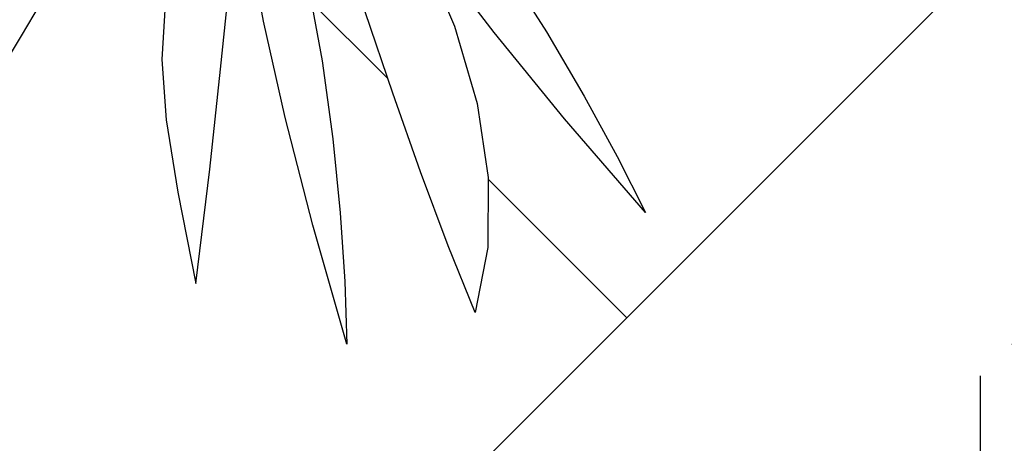
# Model space of a CAD drawing. Units: inches. Extents: x 3590 to 5167, y 65 to 1917.
# Tile 73 of 100: x 5046 to 5065, y 1765 to 1773. Entities that reach past the tile are written whole.
import ezdxf

# ---------------------------------------------------------------- set-up
doc = ezdxf.new("R2010")
doc.units = ezdxf.units.IN
for name, color, linetype, lineweight in [('A-ANNO-DIMS', 2, 'Continuous', 18), ('A-FLOR-PATT', 8, 'Continuous', 13), ('L-PLNT', 94, 'Continuous', 18)]:
    doc.layers.add(name, color=color, linetype=linetype, lineweight=lineweight)
doc.layers.add('DIENHOA', color=3, linetype='Continuous')
doc.styles.get("Standard").update_dxf_attribs({"font": 'arial.ttf'})
doc.dimstyles.new('ISO-25', dxfattribs={"dimtxt": 9, "dimasz": 2.5, "dimexe": 1.25, "dimexo": 0.625, "dimtad": 1, "dimdec": 1, "dimlunit": 3, "dimtxsty": 'Standard', "dimcen": 2.5, "dimadec": 0, "dimazin": 0, "dimtfac": 1, "dimtdec": 1, "dimtmove": 0, "dimatfit": 3, "dimfxl": 1, "dimarcsym": 0})

# ---------------------------------------------------------------- blocks, each defined once
blk = doc.blocks.new('Cay03_mb')
at = {"layer": 'DIENHOA'}
for p, q in [((135.85, -204.28), (162.8, -268.28)), ((113.06, -322.16), (90.79, -256.57)), ((162.8, -268.28), (180.96, -330.4)), ((135.38, -385.56), (113.06, -322.16)), ((180.96, -330.4), (190.01, -389.96)), ((157.6, -444.99), (135.38, -385.56)), ((190.01, -389.96), (189.65, -446.27)), ((179.55, -498.66), (157.6, -444.99)), ((189.65, -446.27), (179.55, -498.66))]:
    blk.add_line(p, q, dxfattribs=at)
for points in [[(23.69, -5.44), (-13.63, -87.94), (-41.14, -152.63), (-59.64, -205.04), (-69.94, -250.66), (-72.84, -295), (-69.17, -343.58), (-59.73, -401.89), (-45.32, -475.45)], [(-45.32, -475.45), (-34.09, -383.24), (-25.4, -302.82), (-18.34, -233.08), (-12.02, -172.9), (-5.55, -121.16), (1.96, -76.75), (11.41, -38.55), (23.69, -5.44)], [(316.49, -418.14), (251.44, -342.76), (194.84, -273.28), (146.52, -210.16), (106.33, -153.83), (74.11, -104.75), (49.71, -63.36), (32.95, -30.11), (23.69, -5.44)], [(23.69, -5.44), (74.94, -57.08), (121.78, -110.58), (164.32, -165.02), (202.67, -219.43), (236.95, -272.89), (267.27, -324.46), (293.75, -373.19), (316.49, -418.14)], [(-276.22, -424.43), (-227.35, -345.43), (-185.71, -276.08), (-150.05, -215.74), (-119.06, -163.76), (-91.49, -119.51), (-66.04, -82.35), (-41.43, -51.64), (-16.39, -26.73)], [(76.25, -524.2), (48.83, -428.48), (26.6, -341.67), (9.22, -264.1), (-3.63, -196.11), (-12.28, -138.04), (-17.07, -90.23), (-18.33, -53.01), (-16.39, -26.73)], [(-16.39, -26.73), (8.47, -95.11), (28.54, -163.33), (44.32, -230.59), (56.3, -296.08), (64.99, -358.99), (70.88, -418.52), (74.46, -473.86), (76.25, -524.2)]]:
    blk.add_lwpolyline(points, dxfattribs=at)
blk = doc.blocks.new('*D322')
at = {"layer": 'A-ANNO-DIMS', "color": 0, "lineweight": -2, "transparency": 16777216}
for p, q in [((5035.744, 1766.184), (5035.744, 1761.199)), ((5064.812, 1766.184), (5064.812, 1761.199)), ((5038.244, 1762.449), (5062.312, 1762.449)), ((5064.812, 1762.449), (5166.991, 1762.449))]:
    blk.add_line(p, q, dxfattribs=at)
at = {"layer": 'A-ANNO-DIMS', "color": 0, "transparency": 16777216}
for points in [[(5038.244, 1762.866), (5038.244, 1762.032), (5035.744, 1762.449)], [(5062.312, 1762.866), (5062.312, 1762.032), (5064.812, 1762.449)]]:
    blk.add_solid(points, dxfattribs=at)
at = {"layer": 'Defpoints', "color": 0, "transparency": 16777216}
for p in [(5035.744, 1766.809), (5064.812, 1766.809), (5064.812, 1762.449)]:
    blk.add_point(p, dxfattribs=at)
at = {"layer": 'A-ANNO-DIMS', "color": 0, "transparency": 16777216, "insert": (5117.152, 1767.669), "char_height": 9, "attachment_point": 5}
blk.add_mtext('PLANT 2\'-5" TYP.', dxfattribs=at)
blk = doc.blocks.new('*D323')
at = {"layer": 'A-ANNO-DIMS', "color": 0, "lineweight": -2, "transparency": 16777216}
for p, q in [((5069.172, 1795.216), (5069.172, 1874.95)), ((5065.437, 1795.216), (5070.422, 1795.216)), ((5069.172, 1769.309), (5069.172, 1792.716)), ((5065.437, 1766.809), (5070.422, 1766.809))]:
    blk.add_line(p, q, dxfattribs=at)
at = {"layer": 'A-ANNO-DIMS', "color": 0, "transparency": 16777216}
for points in [[(5068.756, 1792.716), (5069.589, 1792.716), (5069.172, 1795.216)], [(5068.756, 1769.309), (5069.589, 1769.309), (5069.172, 1766.809)]]:
    blk.add_solid(points, dxfattribs=at)
at = {"layer": 'Defpoints', "color": 0, "transparency": 16777216}
for p in [(5064.812, 1795.216), (5069.172, 1795.216), (5064.812, 1766.809)]:
    blk.add_point(p, dxfattribs=at)
at = {"layer": 'A-ANNO-DIMS', "color": 0, "transparency": 16777216, "insert": (5063.894, 1836.333), "char_height": 9, "attachment_point": 5, "rotation": 90}
blk.add_mtext('2\'-4 1/2" TYP.', dxfattribs=at)

msp = doc.modelspace()

# ---------------------------------------------------------------- hatches: boundary and pattern name
at = {"layer": 'A-FLOR-PATT', "transparency": 33554687}
h = msp.add_hatch(dxfattribs=at)
h.set_pattern_fill('AR-HBONE', color=256, scale=0.2)
h.set_pattern_definition([(45, (-588.972, 0), (0, 28.73682), [60.96, -20.32]), (135, (-574.604, 14.368), (3e-15, 28.73682), [60.96, -20.32])])
h.paths.add_polyline_path([(5071.274, 1796.999), (4933.274, 1796.999), (4933.274, 1753.999), (4962.774, 1753.999, -0.414214), (4928.774, 1719.999), (4933.274, 1718.999), (4933.274, 1334.999), (5071.274, 1334.999)])
h.paths.add_polyline_path([(4951.78, 1521.077), (4951.715, 1521.04), (4951.563, 1520.895)], flags=16)
h.paths.add_polyline_path([(4952.267, 1521.376), (4952.198, 1521.371), (4952.198, 1521.356)], flags=0)
h.paths.add_polyline_path([(4967.051, 1529.728), (4965.231, 1528.694), (4963.411, 1527.714), (4961.756, 1526.851), (4963.589, 1527.449), (4964.036, 1527.478), (4962.975, 1527.249), (4961.76, 1526.852), (4959.792, 1525.834), (4958.005, 1524.895), (4956.24, 1523.93), (4954.504, 1522.919), (4954.129, 1522.682), (4953.361, 1521.997), (4953.366, 1521.998), (4953.605, 1522.064), (4955.106, 1522.761), (4956.921, 1523.434), (4958.678, 1523.915), (4960.358, 1524.2), (4961.945, 1524.286), (4964.171, 1524.108), (4965.958, 1523.309), (4963.863, 1522.976), (4965.187, 1522.499), (4963.366, 1522.497), (4961.545, 1522.487), (4959.764, 1522.461), (4958.304, 1522.419), (4957.974, 1522.388), (4956.307, 1522.232), (4954.718, 1522.071), (4953.251, 1521.899), (4953.525, 1521.623), (4954.331, 1521.379), (4956.243, 1521.23), (4958.039, 1520.93), (4959.684, 1520.483), (4961.16, 1519.896), (4963.107, 1518.8), (4964.393, 1517.325), (4962.973, 1517.726), (4964.558, 1516.661), (4965.407, 1515.708), (4963.507, 1516.322), (4961.68, 1517.005), (4959.935, 1517.745), (4958.282, 1518.528), (4956.732, 1519.343), (4955.295, 1520.175), (4954.672, 1520.572), (4954.513, 1520.627), (4955.658, 1519.318), (4956.703, 1517.982), (4957.644, 1516.647), (4958.485, 1515.334), (4959.55, 1513.524), (4960.438, 1511.769), (4958.841, 1513.62), (4957.452, 1515.325), (4955.819, 1517.459), (4956.665, 1515.448), (4957.111, 1513.923), (4957.447, 1511.714), (4957.076, 1509.793), (4956.538, 1511.11), (4955.992, 1512.569), (4955.444, 1514.125), (4954.898, 1515.735), (4954.357, 1517.356), (4953.824, 1518.943), (4953.305, 1520.452), (4953.065, 1521.116), (4952.971, 1521.146), (4952.949, 1521.086), (4952.73, 1520.199), (4953.37, 1518.024), (4953.757, 1516.373), (4954.051, 1514.765), (4954.264, 1513.221), (4954.471, 1511.131), (4954.497, 1510.402), (4954.409, 1511.76), (4954.264, 1513.221), (4954.051, 1514.765), (4953.757, 1516.373), (4953.37, 1518.024), (4952.877, 1519.698), (4952.716, 1520.141), (4952.533, 1519.059), (4952.374, 1517.789), (4952.219, 1516.312), (4952.046, 1514.6), (4951.833, 1512.626), (4951.557, 1510.363), (4951.203, 1512.168), (4950.852, 1514.339), (4950.985, 1516.376), (4951.66, 1518.286), (4952.593, 1520.481), (4952.357, 1521.13), (4951.855, 1520.328), (4950.839, 1518.908), (4949.777, 1517.587), (4948.916, 1516.617), (4948.111, 1515.256), (4947.089, 1513.554), (4945.889, 1511.615), (4946.326, 1513.402), (4946.562, 1514.249), (4945.528, 1513.327), (4944.581, 1512.531), (4946.018, 1514.508), (4947.204, 1516.048), (4947.893, 1517.313), (4949.307, 1518.764), (4950.414, 1519.767), (4950.451, 1519.806), (4952.267, 1521.376), (4951.645, 1521.493), (4950.404, 1521.18), (4948.044, 1520.359), (4946.119, 1519.452), (4944.572, 1518.475), (4943.35, 1517.443), (4941.997, 1515.92), (4941.661, 1515.275), (4942.813, 1516.99), (4944.572, 1518.475), (4946.119, 1519.452), (4948.044, 1520.359), (4950.404, 1521.18), (4951.645, 1521.493), (4949.647, 1521.868), (4948.6, 1521.756), (4947.126, 1521.57), (4945.42, 1521.348), (4943.45, 1521.105), (4941.183, 1520.856), (4942.86, 1521.613), (4943.873, 1522.03), (4942.952, 1521.909), (4941.41, 1521.485), (4939.543, 1520.67), (4938.968, 1520.226), (4940.733, 1521.299), (4942.952, 1521.909), (4943.702, 1522.008), (4945.894, 1522.7), (4947.565, 1522.714), (4948.921, 1522.566), (4951.131, 1522.183), (4950.971, 1522.297), (4948.129, 1523.006), (4946.035, 1523.707), (4944.232, 1524.521), (4942.707, 1525.461), (4941.444, 1526.537), (4940.43, 1527.761), (4939.649, 1529.143), (4941.421, 1528.122), (4943.147, 1527.132), (4944.841, 1526.175), (4946.514, 1525.25), (4948.179, 1524.359), (4948.365, 1524.263), (4946.475, 1526.045), (4945.181, 1527.54), (4944.19, 1529.033), (4943.496, 1530.54), (4943.278, 1531.36), (4942.498, 1531.919), (4943.114, 1531.762), (4942.959, 1533.659), (4944.14, 1531.989), (4944.612, 1531.323), (4946.202, 1530.463), (4947.486, 1529.509), (4948.79, 1528.226), (4950.368, 1526.237), (4949.485, 1528.155), (4948.851, 1530.123), (4948.491, 1532.041), (4948.381, 1533.918), (4948.501, 1535.76), (4948.827, 1537.573), (4949.418, 1535.565), (4949.957, 1533.569), (4950.464, 1531.586), (4950.961, 1529.617), (4951.391, 1527.954), (4951.724, 1530.687), (4952.201, 1532.58), (4952.889, 1534.33), (4953.77, 1535.951), (4954.827, 1537.46), (4954.521, 1535.39), (4954.273, 1533.937), (4955.58, 1535.663), (4956.748, 1536.739), (4956.159, 1534.78), (4955.589, 1532.873), (4955.043, 1531.006), (4954.525, 1529.166), (4954.038, 1527.341), (4953.638, 1525.733), (4953.611, 1525.586), (4953.398, 1524.166), (4953.382, 1524.009), (4954.07, 1525.476), (4954.912, 1527.022), (4956.136, 1528.894), (4957.847, 1530.577), (4959.376, 1531.54), (4958.256, 1530.104), (4957.143, 1528.663), (4956.066, 1527.243), (4955.056, 1525.871), (4954.141, 1524.571), (4953.352, 1523.372), (4953.311, 1523.303), (4953.273, 1522.925), (4953.261, 1522.382), (4954.103, 1523.373), (4954.63, 1524.284), (4955.961, 1526.358), (4957.23, 1528.13), (4958.421, 1529.609), (4960.037, 1531.368), (4961.374, 1532.375), (4962.101, 1532.77), (4961.07, 1531.061), (4959.987, 1529.438), (4958.869, 1527.908), (4958.15, 1527.007), (4959.803, 1528.003), (4961.589, 1528.793), (4963.391, 1529.328), (4965.211, 1529.632)], flags=16)
h.paths.add_polyline_path([(4962.944, 1523.182), (4961.107, 1523.422), (4960.392, 1523.362), (4962.35, 1523.331)], flags=0)
h.paths.add_polyline_path([(5049.541, 1584.551), (5049.476, 1584.515), (5049.325, 1584.37)], flags=16)
h.paths.add_polyline_path([(5050.028, 1584.851), (5049.959, 1584.845), (5049.959, 1584.83)], flags=0)
h.paths.add_polyline_path([(5042.333, 1581.949), (5043.88, 1582.926), (5045.806, 1583.833), (5048.165, 1584.654), (5049.406, 1584.967), (5047.408, 1585.342), (5046.361, 1585.231), (5044.888, 1585.044), (5043.181, 1584.822), (5041.211, 1584.579), (5038.944, 1584.33), (5040.622, 1585.087), (5041.634, 1585.504), (5040.713, 1585.383), (5039.171, 1584.959), (5037.304, 1584.144), (5036.729, 1583.7), (5038.494, 1584.773), (5040.713, 1585.383), (5041.463, 1585.482), (5043.655, 1586.174), (5045.326, 1586.188), (5046.682, 1586.04), (5048.893, 1585.657), (5048.732, 1585.771), (5045.891, 1586.48), (5043.796, 1587.181), (5041.994, 1587.996), (5040.468, 1588.935), (5039.205, 1590.011), (5038.191, 1591.235), (5037.41, 1592.617), (5039.182, 1591.596), (5040.909, 1590.607), (5042.602, 1589.649), (5044.275, 1588.724), (5045.94, 1587.833), (5046.126, 1587.738), (5044.237, 1589.519), (5042.942, 1591.015), (5041.952, 1592.508), (5041.257, 1594.014), (5041.039, 1594.834), (5040.26, 1595.393), (5040.875, 1595.237), (5040.721, 1597.133), (5041.901, 1595.463), (5042.373, 1594.798), (5043.963, 1593.938), (5045.247, 1592.983), (5046.552, 1591.701), (5048.129, 1589.712), (5047.247, 1591.63), (5046.613, 1593.597), (5046.252, 1595.515), (5046.142, 1597.392), (5046.262, 1599.234), (5046.588, 1601.047), (5047.179, 1599.039), (5047.718, 1597.043), (5048.225, 1595.06), (5048.722, 1593.091), (5049.152, 1591.429), (5049.485, 1594.161), (5049.962, 1596.054), (5050.65, 1597.804), (5051.532, 1599.425), (5052.589, 1600.934), (5052.283, 1598.864), (5052.034, 1597.411), (5053.341, 1599.137), (5054.509, 1600.213), (5053.92, 1598.254), (5053.35, 1596.348), (5052.805, 1594.48), (5052.286, 1592.64), (5051.799, 1590.815), (5051.4, 1589.207), (5051.373, 1589.06), (5051.159, 1587.64), (5051.143, 1587.483), (5051.831, 1588.95), (5052.673, 1590.496), (5053.898, 1592.368), (5055.608, 1594.051), (5057.137, 1595.014), (5056.017, 1593.578), (5054.904, 1592.137), (5053.828, 1590.717), (5052.817, 1589.345), (5051.902, 1588.046), (5051.113, 1586.846), (5051.072, 1586.777), (5051.034, 1586.399), (5051.022, 1585.856), (5051.864, 1586.847), (5052.391, 1587.758), (5053.723, 1589.832), (5054.991, 1591.604), (5056.182, 1593.083), (5057.798, 1594.842), (5059.135, 1595.849), (5059.863, 1596.244), (5058.831, 1594.535), (5057.749, 1592.912), (5056.63, 1591.382), (5055.912, 1590.482), (5057.564, 1591.477), (5059.35, 1592.267), (5061.152, 1592.802), (5062.972, 1593.106), (5064.812, 1593.203), (5062.992, 1592.169), (5061.172, 1591.188), (5059.518, 1590.325), (5061.35, 1590.924), (5061.797, 1590.952), (5060.737, 1590.723), (5059.521, 1590.326), (5057.553, 1589.308), (5055.766, 1588.369), (5054.002, 1587.404), (5052.265, 1586.393), (5051.891, 1586.156), (5051.122, 1585.471), (5051.127, 1585.472), (5051.366, 1585.538), (5052.867, 1586.235), (5054.682, 1586.908), (5056.439, 1587.389), (5058.12, 1587.675), (5059.706, 1587.76), (5061.933, 1587.583), (5063.719, 1586.783), (5061.624, 1586.45), (5062.949, 1585.973), (5061.127, 1585.971), (5059.307, 1585.961), (5057.525, 1585.935), (5056.065, 1585.893), (5055.735, 1585.862), (5054.068, 1585.707), (5052.479, 1585.546), (5051.012, 1585.373), (5051.286, 1585.097), (5052.092, 1584.853), (5054.004, 1584.704), (5055.8, 1584.404), (5057.446, 1583.958), (5058.921, 1583.37), (5060.868, 1582.274), (5062.154, 1580.799), (5060.734, 1581.2), (5062.32, 1580.135), (5063.168, 1579.182), (5061.269, 1579.796), (5059.441, 1580.479), (5057.696, 1581.219), (5056.043, 1582.003), (5054.493, 1582.817), (5053.057, 1583.649), (5052.433, 1584.047), (5052.274, 1584.101), (5053.42, 1582.793), (5054.464, 1581.457), (5055.405, 1580.121), (5056.247, 1578.809), (5057.311, 1576.998), (5058.199, 1575.244), (5056.602, 1577.094), (5055.213, 1578.799), (5053.58, 1580.933), (5054.427, 1578.922), (5054.872, 1577.397), (5055.208, 1575.189), (5054.838, 1573.267), (5054.299, 1574.584), (5053.754, 1576.043), (5053.206, 1577.599), (5052.659, 1579.209), (5052.118, 1580.83), (5051.585, 1582.417), (5051.066, 1583.927), (5050.826, 1584.59), (5050.733, 1584.62), (5050.711, 1584.561), (5050.491, 1583.673), (5051.131, 1581.498), (5051.518, 1579.847), (5051.813, 1578.24), (5052.026, 1576.695), (5052.233, 1574.605), (5052.258, 1573.876), (5052.17, 1575.234), (5052.026, 1576.695), (5051.813, 1578.24), (5051.518, 1579.847), (5051.131, 1581.498), (5050.638, 1583.172), (5050.477, 1583.615), (5050.294, 1582.533), (5050.136, 1581.263), (5049.981, 1579.786), (5049.807, 1578.074), (5049.594, 1576.1), (5049.318, 1573.837), (5048.965, 1575.642), (5048.613, 1577.813), (5048.747, 1579.85), (5049.421, 1581.76), (5050.354, 1583.955), (5050.118, 1584.604), (5049.616, 1583.802), (5048.6, 1582.382), (5047.538, 1581.061), (5046.677, 1580.091), (5045.872, 1578.73), (5044.85, 1577.028), (5043.651, 1575.089), (5044.087, 1576.877), (5044.324, 1577.723), (5043.289, 1576.801), (5042.342, 1576.005), (5043.779, 1577.982), (5044.966, 1579.522), (5045.655, 1580.787), (5047.068, 1582.239), (5048.175, 1583.241), (5048.213, 1583.28), (5050.028, 1584.851), (5049.406, 1584.967), (5048.165, 1584.654), (5045.806, 1583.833), (5043.88, 1582.926), (5042.333, 1581.949), (5041.111, 1580.917), (5039.758, 1579.394), (5039.423, 1578.749), (5040.575, 1580.464)], flags=16)
h.paths.add_polyline_path([(4954.799, 1533.12), (4954.262, 1532.079), (4953.831, 1530.935), (4953.505, 1529.636), (4953.283, 1528.133), (4953.167, 1526.376), (4953.156, 1524.315), (4953.277, 1521.236), (4952.802, 1521.842), (4951.557, 1521.998), (4950.976, 1521.961), (4952.661, 1521.941), (4952.802, 1521.842), (4953.152, 1523.593), (4953.167, 1526.376), (4953.283, 1528.133), (4953.609, 1530.346), (4954.456, 1532.592)], flags=0)
h.paths.add_polyline_path([(5050.563, 1585.316), (5049.318, 1585.472), (5048.737, 1585.435), (5050.422, 1585.415), (5050.563, 1585.316), (5050.914, 1587.067), (5050.928, 1589.851), (5051.045, 1591.607), (5051.371, 1593.82), (5052.217, 1596.066), (5052.56, 1596.594), (5052.024, 1595.554), (5051.592, 1594.409), (5051.266, 1593.11), (5051.045, 1591.607), (5050.928, 1589.851), (5050.918, 1587.789), (5051.038, 1584.71)], flags=0)
h.paths.add_polyline_path([(5058.153, 1586.836), (5060.111, 1586.805), (5060.705, 1586.656), (5058.868, 1586.896)], flags=0)
h.paths.add_polyline_path([(5049.541, 1430.936), (5049.476, 1430.9), (5049.325, 1430.755)], flags=16)
h.paths.add_polyline_path([(5050.028, 1431.236), (5049.959, 1431.231), (5049.959, 1431.215)], flags=0)
h.paths.add_polyline_path([(5046.588, 1447.432), (5047.179, 1445.425), (5047.718, 1443.429), (5048.225, 1441.446), (5048.722, 1439.476), (5049.152, 1437.814), (5049.485, 1440.546), (5049.962, 1442.439), (5050.65, 1444.189), (5051.532, 1445.811), (5052.589, 1447.319), (5052.283, 1445.249), (5052.034, 1443.796), (5053.341, 1445.522), (5054.509, 1446.598), (5053.92, 1444.64), (5053.35, 1442.733), (5052.805, 1440.865), (5052.286, 1439.025), (5051.799, 1437.201), (5051.4, 1435.592), (5051.373, 1435.445), (5051.159, 1434.025), (5051.143, 1433.868), (5051.831, 1435.335), (5052.673, 1436.881), (5053.898, 1438.753), (5055.608, 1440.436), (5057.137, 1441.4), (5056.017, 1439.963), (5054.904, 1438.522), (5053.828, 1437.102), (5052.817, 1435.73), (5051.902, 1434.431), (5051.113, 1433.231), (5051.072, 1433.162), (5051.034, 1432.784), (5051.022, 1432.242), (5051.864, 1433.232), (5052.391, 1434.143), (5053.723, 1436.217), (5054.991, 1437.989), (5056.182, 1439.468), (5057.798, 1441.227), (5059.135, 1442.235), (5059.863, 1442.629), (5058.831, 1440.921), (5057.749, 1439.298), (5056.63, 1437.767), (5055.912, 1436.867), (5057.564, 1437.863), (5059.35, 1438.652), (5061.152, 1439.187), (5062.972, 1439.491), (5064.812, 1439.588), (5062.992, 1438.554), (5061.172, 1437.573), (5059.518, 1436.71), (5061.35, 1437.309), (5061.797, 1437.337), (5060.737, 1437.108), (5059.521, 1436.711), (5057.553, 1435.693), (5055.766, 1434.754), (5054.002, 1433.789), (5052.265, 1432.778), (5051.891, 1432.541), (5051.122, 1431.856), (5051.127, 1431.857), (5051.366, 1431.923), (5052.867, 1432.62), (5054.682, 1433.293), (5056.439, 1433.775), (5058.12, 1434.06), (5059.706, 1434.145), (5061.933, 1433.968), (5063.719, 1433.168), (5061.624, 1432.835), (5062.949, 1432.358), (5061.127, 1432.357), (5059.307, 1432.346), (5057.525, 1432.32), (5056.065, 1432.278), (5055.735, 1432.248), (5054.068, 1432.092), (5052.479, 1431.931), (5051.012, 1431.759), (5051.286, 1431.482), (5052.092, 1431.238), (5054.004, 1431.089), (5055.8, 1430.789), (5057.446, 1430.343), (5058.921, 1429.755), (5060.868, 1428.66), (5062.154, 1427.185), (5060.734, 1427.585), (5062.32, 1426.52), (5063.168, 1425.567), (5061.269, 1426.181), (5059.441, 1426.865), (5057.696, 1427.604), (5056.043, 1428.388), (5054.493, 1429.202), (5053.057, 1430.034), (5052.433, 1430.432), (5052.274, 1430.487), (5053.42, 1429.178), (5054.464, 1427.842), (5055.405, 1426.506), (5056.247, 1425.194), (5057.311, 1423.383), (5058.199, 1421.629), (5056.602, 1423.479), (5055.213, 1425.184), (5053.58, 1427.318), (5054.427, 1425.307), (5054.872, 1423.782), (5055.208, 1421.574), (5054.838, 1419.652), (5054.299, 1420.97), (5053.754, 1422.428), (5053.206, 1423.984), (5052.659, 1425.595), (5052.118, 1427.215), (5051.585, 1428.802), (5051.066, 1430.312), (5050.826, 1430.975), (5050.733, 1431.005), (5050.711, 1430.946), (5050.491, 1430.058), (5051.131, 1427.883), (5051.518, 1426.232), (5051.813, 1424.625), (5052.026, 1423.081), (5052.233, 1420.991), (5052.258, 1420.261), (5052.17, 1421.619), (5052.026, 1423.081), (5051.813, 1424.625), (5051.518, 1426.232), (5051.131, 1427.883), (5050.638, 1429.558), (5050.477, 1430.001), (5050.294, 1428.918), (5050.136, 1427.648), (5049.981, 1426.171), (5049.807, 1424.459), (5049.594, 1422.485), (5049.318, 1420.222), (5048.965, 1422.028), (5048.613, 1424.199), (5048.747, 1426.235), (5049.421, 1428.146), (5050.354, 1430.34), (5050.118, 1430.989), (5049.616, 1430.187), (5048.6, 1428.768), (5047.538, 1427.446), (5046.677, 1426.477), (5045.872, 1425.116), (5044.85, 1423.413), (5043.651, 1421.474), (5044.087, 1423.262), (5044.324, 1424.109), (5043.289, 1423.186), (5042.342, 1422.391), (5043.779, 1424.368), (5044.966, 1425.907), (5045.655, 1427.173), (5047.068, 1428.624), (5048.175, 1429.627), (5048.213, 1429.666), (5050.028, 1431.236), (5049.406, 1431.353), (5048.165, 1431.039), (5045.806, 1430.218), (5043.88, 1429.311), (5042.333, 1428.334), (5041.111, 1427.302), (5039.758, 1425.779), (5039.423, 1425.134), (5040.575, 1426.849), (5042.333, 1428.334), (5043.88, 1429.311), (5045.806, 1430.218), (5048.165, 1431.039), (5049.406, 1431.353), (5047.408, 1431.727), (5046.361, 1431.616), (5044.888, 1431.429), (5043.181, 1431.207), (5041.211, 1430.964), (5038.944, 1430.715), (5040.622, 1431.472), (5041.634, 1431.89), (5040.713, 1431.769), (5039.171, 1431.345), (5037.304, 1430.53), (5036.729, 1430.085), (5038.494, 1431.158), (5040.713, 1431.769), (5041.463, 1431.867), (5043.655, 1432.559), (5045.326, 1432.573), (5046.682, 1432.425), (5048.893, 1432.042), (5048.732, 1432.156), (5045.891, 1432.865), (5043.796, 1433.566), (5041.994, 1434.381), (5040.468, 1435.321), (5039.205, 1436.396), (5038.191, 1437.62), (5037.41, 1439.002), (5039.182, 1437.982), (5040.909, 1436.992), (5042.602, 1436.034), (5044.275, 1435.109), (5045.94, 1434.218), (5046.126, 1434.123), (5044.237, 1435.904), (5042.942, 1437.4), (5041.952, 1438.893), (5041.257, 1440.399), (5041.039, 1441.219), (5040.26, 1441.778), (5040.875, 1441.622), (5040.721, 1443.518), (5041.901, 1441.848), (5042.373, 1441.183), (5043.963, 1440.323), (5045.247, 1439.369), (5046.552, 1438.086), (5048.129, 1436.097), (5047.247, 1438.015), (5046.613, 1439.982), (5046.252, 1441.901), (5046.142, 1443.778), (5046.262, 1445.619)], flags=16)
h.paths.add_polyline_path([(5052.382, 1444.255), (5051.623, 1442.78), (5052.024, 1441.939), (5052.56, 1442.98)], flags=0)
h.paths.add_polyline_path([(5050.563, 1431.701), (5049.318, 1431.857), (5048.737, 1431.821), (5050.422, 1431.8)], flags=0)
h.paths.add_polyline_path([(5058.153, 1433.221), (5060.111, 1433.19), (5060.705, 1433.041), (5058.868, 1433.281)], flags=0)
h.paths.add_polyline_path([(5049.541, 1352.285), (5049.476, 1352.249), (5049.325, 1352.104)], flags=16)
h.paths.add_polyline_path([(5050.028, 1352.585), (5049.959, 1352.58), (5049.959, 1352.564)], flags=0)
h.paths.add_polyline_path([(5046.588, 1368.781), (5047.179, 1366.774), (5047.718, 1364.778), (5048.225, 1362.795), (5048.722, 1360.825), (5049.152, 1359.163), (5049.485, 1361.896), (5049.962, 1363.789), (5050.65, 1365.538), (5051.532, 1367.16), (5052.589, 1368.669), (5052.283, 1366.598), (5052.034, 1365.145), (5053.341, 1366.871), (5054.509, 1367.947), (5053.92, 1365.989), (5053.35, 1364.082), (5052.805, 1362.214), (5052.286, 1360.374), (5051.799, 1358.55), (5051.4, 1356.942), (5051.373, 1356.794), (5051.159, 1355.374), (5051.143, 1355.218), (5051.831, 1356.684), (5052.673, 1358.23), (5053.898, 1360.102), (5055.608, 1361.786), (5057.137, 1362.749), (5056.017, 1361.313), (5054.904, 1359.872), (5053.828, 1358.452), (5052.817, 1357.079), (5051.902, 1355.78), (5051.113, 1354.581), (5051.072, 1354.512), (5051.034, 1354.133), (5051.022, 1353.591), (5051.864, 1354.581), (5052.391, 1355.492), (5053.723, 1357.566), (5054.991, 1359.338), (5056.182, 1360.817), (5057.798, 1362.577), (5059.135, 1363.584), (5059.863, 1363.979), (5058.831, 1362.27), (5057.749, 1360.647), (5056.63, 1359.117), (5055.912, 1358.216), (5057.564, 1359.212), (5059.35, 1360.001), (5061.152, 1360.536), (5062.972, 1360.841), (5064.812, 1360.937), (5062.992, 1359.903), (5061.172, 1358.923), (5059.518, 1358.059), (5061.35, 1358.658), (5061.797, 1358.687), (5060.737, 1358.458), (5059.521, 1358.061), (5057.553, 1357.043), (5055.766, 1356.103), (5054.002, 1355.138), (5052.265, 1354.127), (5051.891, 1353.89), (5051.122, 1353.206), (5051.127, 1353.206), (5051.366, 1353.272), (5052.867, 1353.969), (5054.682, 1354.643), (5056.439, 1355.124), (5058.12, 1355.409), (5059.706, 1355.495), (5061.933, 1355.317), (5063.719, 1354.518), (5061.624, 1354.184), (5062.949, 1353.708), (5061.127, 1353.706), (5059.307, 1353.695), (5057.525, 1353.669), (5056.065, 1353.627), (5055.735, 1353.597), (5054.068, 1353.441), (5052.479, 1353.28), (5051.012, 1353.108), (5051.286, 1352.831), (5052.092, 1352.587), (5054.004, 1352.439), (5055.8, 1352.138), (5057.446, 1351.692), (5058.921, 1351.104), (5060.868, 1350.009), (5062.154, 1348.534), (5060.734, 1348.935), (5062.32, 1347.869), (5063.168, 1346.916), (5061.269, 1347.53), (5059.441, 1348.214), (5057.696, 1348.954), (5056.043, 1349.737), (5054.493, 1350.551), (5053.057, 1351.383), (5052.433, 1351.781), (5052.274, 1351.836), (5053.42, 1350.527), (5054.464, 1349.191), (5055.405, 1347.855), (5056.247, 1346.543), (5057.311, 1344.733), (5058.199, 1342.978), (5056.602, 1344.828), (5055.213, 1346.534), (5053.58, 1348.667), (5054.427, 1346.656), (5054.872, 1345.132), (5055.208, 1342.923), (5054.838, 1341.002), (5054.299, 1342.319), (5053.754, 1343.778), (5053.206, 1345.334), (5052.659, 1346.944), (5052.118, 1348.564), (5051.585, 1350.151), (5051.066, 1351.661), (5050.826, 1352.324), (5050.733, 1352.355), (5050.711, 1352.295), (5050.491, 1351.408), (5051.131, 1349.232), (5051.518, 1347.581), (5051.813, 1345.974), (5052.026, 1344.43), (5052.233, 1342.34), (5052.258, 1341.61), (5052.17, 1342.969), (5052.026, 1344.43), (5051.813, 1345.974), (5051.518, 1347.581), (5051.131, 1349.232), (5050.638, 1350.907), (5050.477, 1351.35), (5050.294, 1350.267), (5050.136, 1348.997), (5049.981, 1347.52), (5049.807, 1345.809), (5049.594, 1343.835), (5049.318, 1341.571), (5048.965, 1343.377), (5048.613, 1345.548), (5048.747, 1347.585), (5049.421, 1349.495), (5050.354, 1351.689), (5050.118, 1352.339), (5049.616, 1351.536), (5048.6, 1350.117), (5047.538, 1348.795), (5046.677, 1347.826), (5045.872, 1346.465), (5044.85, 1344.763), (5043.651, 1342.824), (5044.087, 1344.611), (5044.324, 1345.458), (5043.289, 1344.535), (5042.342, 1343.74), (5043.779, 1345.717), (5044.966, 1347.256), (5045.655, 1348.522), (5047.068, 1349.973), (5048.175, 1350.976), (5048.213, 1351.015), (5050.028, 1352.585), (5049.406, 1352.702), (5048.165, 1352.388), (5045.806, 1351.567), (5043.88, 1350.661), (5042.333, 1349.683), (5041.111, 1348.651), (5039.758, 1347.128), (5039.423, 1346.483), (5040.575, 1348.198), (5042.333, 1349.683), (5043.88, 1350.661), (5045.806, 1351.567), (5048.165, 1352.388), (5049.406, 1352.702), (5047.408, 1353.076), (5046.361, 1352.965), (5044.888, 1352.779), (5043.181, 1352.556), (5041.211, 1352.313), (5038.944, 1352.065), (5040.622, 1352.821), (5041.634, 1353.239), (5040.713, 1353.118), (5039.171, 1352.694), (5037.304, 1351.879), (5036.729, 1351.434), (5038.494, 1352.508), (5040.713, 1353.118), (5041.463, 1353.216), (5043.655, 1353.909), (5045.326, 1353.923), (5046.682, 1353.774), (5048.893, 1353.391), (5048.732, 1353.506), (5045.891, 1354.214), (5043.796, 1354.915), (5041.994, 1355.73), (5040.468, 1356.67), (5039.205, 1357.746), (5038.191, 1358.969), (5037.41, 1360.352), (5039.182, 1359.331), (5040.909, 1358.341), (5042.602, 1357.383), (5044.275, 1356.458), (5045.94, 1355.567), (5046.126, 1355.472), (5044.237, 1357.253), (5042.942, 1358.749), (5041.952, 1360.242), (5041.257, 1361.748), (5041.039, 1362.568), (5040.26, 1363.128), (5040.875, 1362.971), (5040.721, 1364.867), (5041.901, 1363.197), (5042.373, 1362.532), (5043.963, 1361.672), (5045.247, 1360.718), (5046.552, 1359.435), (5048.129, 1357.446), (5047.247, 1359.364), (5046.613, 1361.331), (5046.252, 1363.25), (5046.142, 1365.127), (5046.262, 1366.969)], flags=16)
h.paths.add_polyline_path([(5052.382, 1365.604), (5051.623, 1364.129), (5052.024, 1363.288), (5052.56, 1364.329)], flags=0)
h.paths.add_polyline_path([(4951.78, 1698.041), (4951.715, 1698.005), (4951.563, 1697.859)], flags=16)
h.paths.add_polyline_path([(4952.267, 1698.341), (4952.198, 1698.335), (4952.198, 1698.32)], flags=0)
h.paths.add_polyline_path([(4957.076, 1686.757), (4956.538, 1688.074), (4955.992, 1689.533), (4955.444, 1691.089), (4954.898, 1692.699), (4954.357, 1694.32), (4953.824, 1695.907), (4953.305, 1697.417), (4953.065, 1698.08), (4952.971, 1698.11), (4952.949, 1698.051), (4952.73, 1697.163), (4953.37, 1694.988), (4953.757, 1693.337), (4954.051, 1691.729), (4954.264, 1690.185), (4954.471, 1688.095), (4954.497, 1687.366), (4954.409, 1688.724), (4954.264, 1690.185), (4954.051, 1691.729), (4953.757, 1693.337), (4953.37, 1694.988), (4952.877, 1696.662), (4952.716, 1697.105), (4952.533, 1696.023), (4952.374, 1694.753), (4952.219, 1693.276), (4952.046, 1691.564), (4951.833, 1689.59), (4951.557, 1687.327), (4951.203, 1689.132), (4950.852, 1691.303), (4950.985, 1693.34), (4951.66, 1695.25), (4952.593, 1697.445), (4952.357, 1698.094), (4951.855, 1697.292), (4950.839, 1695.872), (4949.777, 1694.551), (4948.916, 1693.581), (4948.111, 1692.22), (4947.089, 1690.518), (4945.889, 1688.579), (4946.326, 1690.366), (4946.562, 1691.213), (4945.528, 1690.291), (4944.581, 1689.495), (4946.018, 1691.472), (4947.204, 1693.012), (4947.893, 1694.277), (4949.307, 1695.729), (4950.414, 1696.731), (4950.451, 1696.77), (4952.267, 1698.341), (4951.645, 1698.457), (4950.404, 1698.144), (4948.044, 1697.323), (4946.119, 1696.416), (4944.572, 1695.439), (4943.35, 1694.407), (4941.997, 1692.884), (4941.661, 1692.239), (4942.813, 1693.954), (4944.572, 1695.439), (4946.119, 1696.416), (4948.044, 1697.323), (4950.404, 1698.144), (4951.645, 1698.457), (4949.647, 1698.832), (4948.6, 1698.72), (4947.126, 1698.534), (4945.42, 1698.312), (4943.45, 1698.069), (4941.183, 1697.82), (4942.86, 1698.577), (4943.873, 1698.994), (4942.952, 1698.873), (4941.41, 1698.449), (4939.543, 1697.634), (4938.968, 1697.19), (4940.733, 1698.263), (4942.952, 1698.873), (4943.702, 1698.972), (4945.894, 1699.664), (4947.565, 1699.678), (4948.921, 1699.53), (4951.131, 1699.147), (4950.971, 1699.261), (4948.129, 1699.97), (4946.035, 1700.671), (4944.232, 1701.486), (4942.707, 1702.425), (4941.444, 1703.501), (4940.43, 1704.725), (4939.649, 1706.107), (4941.421, 1705.086), (4943.147, 1704.097), (4944.841, 1703.139), (4946.514, 1702.214), (4948.179, 1701.323), (4948.365, 1701.227), (4946.475, 1703.009), (4945.181, 1704.505), (4944.19, 1705.997), (4943.496, 1707.504), (4943.278, 1708.324), (4942.498, 1708.883), (4943.114, 1708.727), (4942.959, 1710.623), (4944.14, 1708.953), (4944.612, 1708.287), (4946.202, 1707.428), (4947.486, 1706.473), (4948.79, 1705.191), (4950.368, 1703.202), (4949.485, 1705.12), (4948.851, 1707.087), (4948.491, 1709.005), (4948.381, 1710.882), (4948.501, 1712.724), (4948.827, 1714.537), (4949.418, 1712.529), (4949.957, 1710.533), (4950.464, 1708.55), (4950.961, 1706.581), (4951.391, 1704.919), (4951.724, 1707.651), (4952.201, 1709.544), (4952.889, 1711.294), (4953.77, 1712.915), (4954.827, 1714.424), (4954.521, 1712.354), (4954.273, 1710.901), (4955.58, 1712.627), (4956.748, 1713.703), (4956.159, 1711.744), (4955.589, 1709.837), (4955.043, 1707.97), (4954.525, 1706.13), (4954.038, 1704.305), (4953.638, 1702.697), (4953.611, 1702.55), (4953.398, 1701.13), (4953.382, 1700.973), (4954.07, 1702.44), (4954.912, 1703.986), (4956.136, 1705.858), (4957.847, 1707.541), (4959.376, 1708.504), (4958.256, 1707.068), (4957.143, 1705.627), (4956.066, 1704.207), (4955.056, 1702.835), (4954.141, 1701.536), (4953.352, 1700.336), (4953.311, 1700.267), (4953.273, 1699.889), (4953.261, 1699.346), (4954.103, 1700.337), (4954.63, 1701.248), (4955.961, 1703.322), (4957.23, 1705.094), (4958.421, 1706.573), (4960.037, 1708.332), (4961.374, 1709.339), (4962.101, 1709.734), (4961.07, 1708.025), (4959.987, 1706.402), (4958.869, 1704.872), (4958.15, 1703.972), (4959.803, 1704.967), (4961.589, 1705.757), (4963.391, 1706.292), (4965.211, 1706.596), (4967.051, 1706.692), (4965.231, 1705.659), (4963.411, 1704.678), (4961.756, 1703.815), (4963.589, 1704.413), (4964.036, 1704.442), (4962.975, 1704.213), (4961.76, 1703.816), (4959.792, 1702.798), (4958.005, 1701.859), (4956.24, 1700.894), (4954.504, 1699.883), (4954.129, 1699.646), (4953.361, 1698.961), (4953.366, 1698.962), (4953.605, 1699.028), (4955.106, 1699.725), (4956.921, 1700.398), (4958.678, 1700.879), (4960.358, 1701.164), (4961.945, 1701.25), (4964.171, 1701.073), (4965.958, 1700.273), (4963.863, 1699.94), (4965.187, 1699.463), (4963.366, 1699.461), (4961.545, 1699.451), (4959.764, 1699.425), (4958.304, 1699.383), (4957.974, 1699.352), (4956.307, 1699.197), (4954.718, 1699.036), (4953.251, 1698.863), (4953.525, 1698.587), (4954.331, 1698.343), (4956.243, 1698.194), (4958.039, 1697.894), (4959.684, 1697.447), (4961.16, 1696.86), (4963.107, 1695.764), (4964.393, 1694.289), (4962.973, 1694.69), (4964.558, 1693.625), (4965.407, 1692.672), (4963.507, 1693.286), (4961.68, 1693.969), (4959.935, 1694.709), (4958.282, 1695.492), (4956.732, 1696.307), (4955.295, 1697.139), (4954.672, 1697.536), (4954.513, 1697.591), (4955.658, 1696.282), (4956.703, 1694.946), (4957.644, 1693.611), (4958.485, 1692.298), (4959.55, 1690.488), (4960.438, 1688.733), (4958.841, 1690.584), (4957.452, 1692.289), (4955.819, 1694.423), (4956.665, 1692.412), (4957.111, 1690.887), (4957.447, 1688.678)], flags=16)
h.paths.add_polyline_path([(5050.563, 1353.05), (5049.318, 1353.207), (5048.737, 1353.17), (5050.422, 1353.15)], flags=0)
h.paths.add_polyline_path([(4951.78, 1351.486), (4951.715, 1351.45), (4951.563, 1351.305)], flags=16)
h.paths.add_polyline_path([(4952.267, 1351.786), (4952.198, 1351.78), (4952.198, 1351.765)], flags=0)
h.paths.add_polyline_path([(4954.827, 1367.869), (4954.521, 1365.799), (4954.273, 1364.346), (4955.58, 1366.072), (4956.748, 1367.148), (4956.159, 1365.19), (4955.589, 1363.283), (4955.043, 1361.415), (4954.525, 1359.575), (4954.038, 1357.751), (4953.638, 1356.142), (4953.611, 1355.995), (4953.398, 1354.575), (4953.382, 1354.418), (4954.07, 1355.885), (4954.912, 1357.431), (4956.136, 1359.303), (4957.847, 1360.986), (4959.376, 1361.95), (4958.256, 1360.513), (4957.143, 1359.072), (4956.066, 1357.652), (4955.056, 1356.28), (4954.141, 1354.981), (4953.352, 1353.781), (4953.311, 1353.712), (4953.273, 1353.334), (4953.261, 1352.792), (4954.103, 1353.782), (4954.63, 1354.693), (4955.961, 1356.767), (4957.23, 1358.539), (4958.421, 1360.018), (4960.037, 1361.777), (4961.374, 1362.785), (4962.101, 1363.179), (4961.07, 1361.471), (4959.987, 1359.848), (4958.869, 1358.317), (4958.15, 1357.417), (4959.803, 1358.413), (4961.589, 1359.202), (4963.391, 1359.737), (4965.211, 1360.041), (4967.051, 1360.138), (4965.231, 1359.104), (4963.411, 1358.123), (4961.756, 1357.26), (4963.589, 1357.859), (4964.036, 1357.887), (4962.975, 1357.658), (4961.76, 1357.261), (4959.792, 1356.243), (4958.005, 1355.304), (4956.24, 1354.339), (4954.504, 1353.328), (4954.129, 1353.091), (4953.361, 1352.406), (4953.366, 1352.407), (4953.605, 1352.473), (4955.106, 1353.17), (4956.921, 1353.843), (4958.678, 1354.325), (4960.358, 1354.61), (4961.945, 1354.695), (4964.171, 1354.518), (4965.958, 1353.718), (4963.863, 1353.385), (4965.187, 1352.908), (4963.366, 1352.907), (4961.545, 1352.896), (4959.764, 1352.87), (4958.304, 1352.828), (4957.974, 1352.798), (4956.307, 1352.642), (4954.718, 1352.481), (4953.251, 1352.309), (4953.525, 1352.032), (4954.331, 1351.788), (4956.243, 1351.639), (4958.039, 1351.339), (4959.684, 1350.893), (4961.16, 1350.305), (4963.107, 1349.21), (4964.393, 1347.735), (4962.973, 1348.135), (4964.558, 1347.07), (4965.407, 1346.117), (4963.507, 1346.731), (4961.68, 1347.414), (4959.935, 1348.154), (4958.282, 1348.938), (4956.732, 1349.752), (4955.295, 1350.584), (4954.672, 1350.982), (4954.513, 1351.036), (4955.658, 1349.728), (4956.703, 1348.392), (4957.644, 1347.056), (4958.485, 1345.744), (4959.55, 1343.933), (4960.438, 1342.179), (4958.841, 1344.029), (4957.452, 1345.734), (4955.819, 1347.868), (4956.665, 1345.857), (4957.111, 1344.332), (4957.447, 1342.124), (4957.076, 1340.202), (4956.538, 1341.52), (4955.992, 1342.978), (4955.444, 1344.534), (4954.898, 1346.145), (4954.357, 1347.765), (4953.824, 1349.352), (4953.305, 1350.862), (4953.065, 1351.525), (4952.971, 1351.555), (4952.949, 1351.496), (4952.73, 1350.608), (4953.37, 1348.433), (4953.757, 1346.782), (4954.051, 1345.175), (4954.264, 1343.631), (4954.471, 1341.541), (4954.497, 1340.811), (4954.409, 1342.169), (4954.264, 1343.631), (4954.051, 1345.175), (4953.757, 1346.782), (4953.37, 1348.433), (4952.877, 1350.108), (4952.716, 1350.551), (4952.533, 1349.468), (4952.374, 1348.198), (4952.219, 1346.721), (4952.046, 1345.009), (4951.833, 1343.035), (4951.557, 1340.772), (4951.203, 1342.578), (4950.852, 1344.749), (4950.985, 1346.785), (4951.66, 1348.696), (4952.593, 1350.89), (4952.357, 1351.539), (4951.855, 1350.737), (4950.839, 1349.318), (4949.777, 1347.996), (4948.916, 1347.027), (4948.111, 1345.665), (4947.089, 1343.963), (4945.889, 1342.024), (4946.326, 1343.812), (4946.562, 1344.659), (4945.528, 1343.736), (4944.581, 1342.941), (4946.018, 1344.918), (4947.204, 1346.457), (4947.893, 1347.723), (4949.307, 1349.174), (4950.414, 1350.177), (4950.451, 1350.216), (4952.267, 1351.786), (4951.645, 1351.903), (4950.404, 1351.589), (4948.044, 1350.768), (4946.119, 1349.861), (4944.572, 1348.884), (4943.35, 1347.852), (4941.997, 1346.329), (4941.661, 1345.684), (4942.813, 1347.399), (4944.572, 1348.884), (4946.119, 1349.861), (4948.044, 1350.768), (4950.404, 1351.589), (4951.645, 1351.903), (4949.647, 1352.277), (4948.6, 1352.166), (4947.126, 1351.979), (4945.42, 1351.757), (4943.45, 1351.514), (4941.183, 1351.265), (4942.86, 1352.022), (4943.873, 1352.44), (4942.952, 1352.319), (4941.41, 1351.895), (4939.543, 1351.08), (4938.968, 1350.635), (4940.733, 1351.708), (4942.952, 1352.319), (4943.702, 1352.417), (4945.894, 1353.109), (4947.565, 1353.123), (4948.921, 1352.975), (4951.131, 1352.592), (4950.971, 1352.706), (4948.129, 1353.415), (4946.035, 1354.116), (4944.232, 1354.931), (4942.707, 1355.871), (4941.444, 1356.946), (4940.43, 1358.17), (4939.649, 1359.552), (4941.421, 1358.532), (4943.147, 1357.542), (4944.841, 1356.584), (4946.514, 1355.659), (4948.179, 1354.768), (4948.365, 1354.673), (4946.475, 1356.454), (4945.181, 1357.95), (4944.19, 1359.443), (4943.496, 1360.949), (4943.278, 1361.769), (4942.498, 1362.328), (4943.114, 1362.172), (4942.959, 1364.068), (4944.14, 1362.398), (4944.612, 1361.733), (4946.202, 1360.873), (4947.486, 1359.919), (4948.79, 1358.636), (4950.368, 1356.647), (4949.485, 1358.565), (4948.851, 1360.532), (4948.491, 1362.451), (4948.381, 1364.328), (4948.501, 1366.169), (4948.827, 1367.982), (4949.418, 1365.975), (4949.957, 1363.979), (4950.464, 1361.995), (4950.961, 1360.026), (4951.391, 1358.364), (4951.724, 1361.096), (4952.201, 1362.989), (4952.889, 1364.739), (4953.77, 1366.361)], flags=16)
h.paths.add_polyline_path([(4954.799, 1363.53), (4954.262, 1362.489), (4953.831, 1361.344), (4953.505, 1360.045), (4953.283, 1358.543), (4953.167, 1356.786), (4953.156, 1354.724), (4953.277, 1351.646), (4952.802, 1352.251), (4951.557, 1352.407), (4950.976, 1352.371), (4952.661, 1352.35), (4952.802, 1352.251), (4953.152, 1354.002), (4953.167, 1356.786), (4953.283, 1358.543), (4953.609, 1360.755), (4954.456, 1363.001)], flags=0)
h.paths.add_polyline_path([(4952.802, 1698.806), (4951.557, 1698.962), (4950.976, 1698.925), (4952.661, 1698.905), (4952.802, 1698.806), (4953.152, 1700.557), (4953.167, 1703.34), (4953.283, 1705.097), (4953.609, 1707.31), (4954.456, 1709.556), (4954.799, 1710.084), (4954.262, 1709.043), (4953.831, 1707.899), (4953.505, 1706.6), (4953.283, 1705.097), (4953.167, 1703.34), (4953.156, 1701.279), (4953.277, 1698.2)], flags=0)
h.paths.add_polyline_path([(4962.944, 1700.146), (4961.107, 1700.386), (4960.392, 1700.326), (4962.35, 1700.295)], flags=0)
h.paths.add_polyline_path([(5058.153, 1354.57), (5060.111, 1354.539), (5060.705, 1354.391), (5058.868, 1354.631)], flags=0)
h.paths.add_polyline_path([(4962.944, 1353.591), (4961.107, 1353.831), (4960.392, 1353.771), (4962.35, 1353.74)], flags=0)
h.paths.add_polyline_path([(5049.541, 1778.72), (5049.476, 1778.684), (5049.325, 1778.539)], flags=16)
h.paths.add_polyline_path([(5050.028, 1779.02), (5049.959, 1779.014), (5049.959, 1778.999)], flags=0)
h.paths.add_polyline_path([(5052.258, 1768.045), (5052.17, 1769.403), (5052.026, 1770.864), (5051.813, 1772.409), (5051.518, 1774.016), (5051.131, 1775.667), (5050.638, 1777.341), (5050.477, 1777.784), (5050.294, 1776.702), (5050.136, 1775.432), (5049.981, 1773.955), (5049.807, 1772.243), (5049.594, 1770.269), (5049.318, 1768.006), (5048.965, 1769.811), (5048.613, 1771.982), (5048.747, 1774.019), (5049.421, 1775.929), (5050.354, 1778.124), (5050.118, 1778.773), (5049.616, 1777.971), (5048.6, 1776.551), (5047.538, 1775.23), (5046.677, 1774.26), (5045.872, 1772.899), (5044.85, 1771.197), (5043.651, 1769.258), (5044.087, 1771.046), (5044.324, 1771.892), (5043.289, 1770.97), (5042.342, 1770.174), (5043.779, 1772.151), (5044.966, 1773.691), (5045.655, 1774.956), (5047.068, 1776.408), (5048.175, 1777.41), (5048.213, 1777.449), (5050.028, 1779.02), (5049.406, 1779.136), (5048.165, 1778.823), (5045.806, 1778.002), (5043.88, 1777.095), (5042.333, 1776.118), (5041.111, 1775.086), (5039.758, 1773.563), (5039.423, 1772.918), (5040.575, 1774.633), (5042.333, 1776.118), (5043.88, 1777.095), (5045.806, 1778.002), (5048.165, 1778.823), (5049.406, 1779.136), (5047.408, 1779.511), (5046.361, 1779.4), (5044.888, 1779.213), (5043.181, 1778.991), (5041.211, 1778.748), (5038.944, 1778.499), (5040.622, 1779.256), (5041.634, 1779.673), (5040.713, 1779.552), (5039.171, 1779.128), (5037.304, 1778.313), (5036.729, 1777.869), (5038.494, 1778.942), (5040.713, 1779.552), (5041.463, 1779.651), (5043.655, 1780.343), (5045.326, 1780.357), (5046.682, 1780.209), (5048.893, 1779.826), (5048.732, 1779.94), (5045.891, 1780.649), (5043.796, 1781.35), (5041.994, 1782.165), (5040.468, 1783.104), (5039.205, 1784.18), (5038.191, 1785.404), (5037.41, 1786.786), (5039.182, 1785.765), (5040.909, 1784.776), (5042.602, 1783.818), (5044.275, 1782.893), (5045.94, 1782.002), (5046.126, 1781.907), (5044.237, 1783.688), (5042.942, 1785.184), (5041.952, 1786.677), (5041.257, 1788.183), (5041.039, 1789.003), (5040.26, 1789.562), (5040.875, 1789.406), (5040.721, 1791.302), (5041.901, 1789.632), (5042.373, 1788.967), (5043.963, 1788.107), (5045.247, 1787.152), (5046.552, 1785.87), (5048.129, 1783.881), (5047.247, 1785.799), (5046.613, 1787.766), (5046.252, 1789.684), (5046.142, 1791.561), (5046.262, 1793.403), (5046.588, 1795.216), (5047.179, 1793.208), (5047.718, 1791.213), (5048.225, 1789.229), (5048.722, 1787.26), (5049.152, 1785.598), (5049.485, 1788.33), (5049.962, 1790.223), (5050.65, 1791.973), (5051.532, 1793.594), (5052.589, 1795.103), (5052.283, 1793.033), (5052.034, 1791.58), (5053.341, 1793.306), (5054.509, 1794.382), (5053.92, 1792.423), (5053.35, 1790.517), (5052.805, 1788.649), (5052.286, 1786.809), (5051.799, 1784.984), (5051.4, 1783.376), (5051.373, 1783.229), (5051.159, 1781.809), (5051.143, 1781.652), (5051.831, 1783.119), (5052.673, 1784.665), (5053.898, 1786.537), (5055.608, 1788.22), (5057.137, 1789.183), (5056.017, 1787.747), (5054.904, 1786.306), (5053.828, 1784.886), (5052.817, 1783.514), (5051.902, 1782.215), (5051.113, 1781.015), (5051.072, 1780.946), (5051.034, 1780.568), (5051.022, 1780.025), (5051.864, 1781.016), (5052.391, 1781.927), (5053.723, 1784.001), (5054.991, 1785.773), (5056.182, 1787.252), (5057.798, 1789.011), (5059.135, 1790.018), (5059.863, 1790.413), (5058.831, 1788.704), (5057.749, 1787.081), (5056.63, 1785.551), (5055.912, 1784.651), (5057.564, 1785.646), (5059.35, 1786.436), (5061.152, 1786.971), (5062.972, 1787.275), (5064.812, 1787.372), (5062.992, 1786.338), (5061.172, 1785.357), (5059.518, 1784.494), (5061.35, 1785.093), (5061.797, 1785.121), (5060.737, 1784.892), (5059.521, 1784.495), (5057.553, 1783.477), (5055.766, 1782.538), (5054.002, 1781.573), (5052.265, 1780.562), (5051.891, 1780.325), (5051.122, 1779.64), (5051.127, 1779.641), (5051.366, 1779.707), (5052.867, 1780.404), (5054.682, 1781.077), (5056.439, 1781.558), (5058.12, 1781.844), (5059.706, 1781.929), (5061.933, 1781.752), (5063.719, 1780.952), (5061.624, 1780.619), (5062.949, 1780.142), (5061.127, 1780.14), (5059.307, 1780.13), (5057.525, 1780.104), (5056.065, 1780.062), (5055.735, 1780.031), (5054.068, 1779.876), (5052.479, 1779.715), (5051.012, 1779.542), (5051.286, 1779.266), (5052.092, 1779.022), (5054.004, 1778.873), (5055.8, 1778.573), (5057.446, 1778.127), (5058.921, 1777.539), (5060.868, 1776.443), (5062.154, 1774.968), (5060.734, 1775.369), (5062.32, 1774.304), (5063.168, 1773.351), (5061.269, 1773.965), (5059.441, 1774.648), (5057.696, 1775.388), (5056.043, 1776.172), (5054.493, 1776.986), (5053.057, 1777.818), (5052.433, 1778.216), (5052.274, 1778.27), (5053.42, 1776.962), (5054.464, 1775.626), (5055.405, 1774.29), (5056.247, 1772.978), (5057.311, 1771.167), (5058.199, 1769.413), (5056.602, 1771.263), (5055.213, 1772.968), (5053.58, 1775.102), (5054.427, 1773.091), (5054.872, 1771.566), (5055.208, 1769.358), (5054.838, 1767.436), (5054.299, 1768.753), (5053.754, 1770.212), (5053.206, 1771.768), (5052.659, 1773.378), (5052.118, 1774.999), (5051.585, 1776.586), (5051.066, 1778.096), (5050.826, 1778.759), (5050.733, 1778.789), (5050.711, 1778.73), (5050.491, 1777.842), (5051.131, 1775.667), (5051.518, 1774.016), (5051.813, 1772.409), (5052.026, 1770.864), (5052.233, 1768.774)], flags=16)
h.paths.add_polyline_path([(5050.563, 1779.485), (5049.318, 1779.641), (5048.737, 1779.604), (5050.422, 1779.584), (5050.563, 1779.485), (5050.914, 1781.236), (5050.928, 1784.02), (5051.045, 1785.776), (5051.371, 1787.989), (5052.217, 1790.235), (5052.56, 1790.763), (5052.024, 1789.723), (5051.592, 1788.578), (5051.266, 1787.279), (5051.045, 1785.776), (5050.928, 1784.02), (5050.918, 1781.958), (5051.038, 1778.879)], flags=0)
h.paths.add_polyline_path([(5058.153, 1781.005), (5060.111, 1780.974), (5060.705, 1780.825), (5058.868, 1781.065)], flags=0)

# ---------------------------------------------------------------- block references
at = {"layer": 'L-PLNT', "xscale": 0.0245452446402784, "yscale": 0.0245452446402784, "zscale": 0.0245452446402784}
msp.add_blockref('Cay03_mb', (5050.431, 1779.676), dxfattribs=at)

# ---------------------------------------------------------------- dimensions: what is measured, and where the dimension line sits
at = {"layer": 'A-ANNO-DIMS'}
dim = msp.add_linear_dim(base=(5069.172, 1795.216), p1=(5064.812, 1766.809), p2=(5064.812, 1795.216), angle=90, text='<> TYP.', dimstyle='ISO-25', override={"dimdec": 1, "dimlfac": 1, "dimrnd": 0, "dimzin": 1, "dimdsep": 46, "dimlunit": 4, "dimfrac": 2}, dxfattribs=at)
dim.commit()
dim.dimension.update_dxf_attribs({"geometry": '*D323', "text_midpoint": (5063.894, 1836.333)})
dim = msp.add_linear_dim(base=(5064.812, 1762.449), p1=(5035.744, 1766.809), p2=(5064.812, 1766.809), text='PLANT <> TYP.', dimstyle='ISO-25', override={"dimdec": 1, "dimlfac": 1, "dimrnd": 0, "dimzin": 1, "dimdsep": 46, "dimlunit": 4, "dimfrac": 2}, dxfattribs=at)
dim.commit()
dim.dimension.update_dxf_attribs({"geometry": '*D322', "text_midpoint": (5117.152, 1767.669)})

doc.saveas('drawing.dxf')
